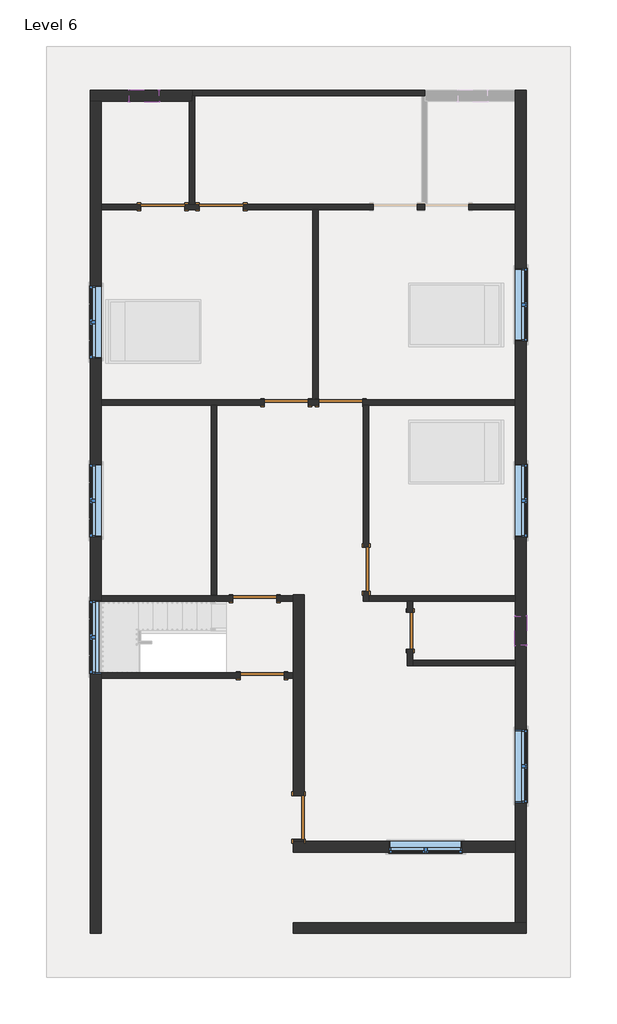
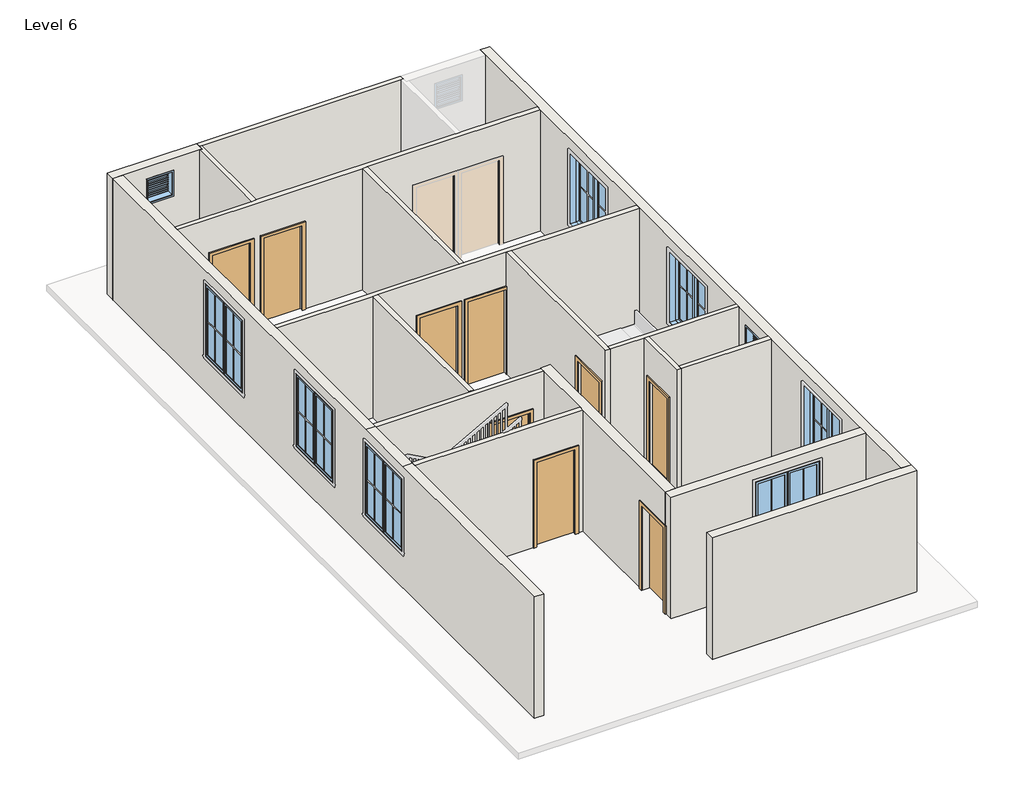
# One storey, part 1 of 3: 18 walls, 9 doors, 9 windows.
"""IFC4 building model written with IfcOpenShell, lengths in millimetres."""

from ifc_helpers import new_model, si_unit, frame, origin, place, context, project, spatial, polyline, outline, extrude, faceted_brep, transform, mapped, element, save
from components import door_78caadf7, single_flush_door_3_e5f9f3c4, single_flush_door_3_305aa2a5, single_flush_door_3_0ca8825f, window_casement_double_win_5_f93960c7, window_f2d8fef0

model = new_model("IFC4")

# Units and contexts
model_context = context("Model", 3, world=origin())
ifc_project = project(units=[si_unit("LENGTHUNIT", "METRE", prefix="MILLI")], contexts=[model_context])

# Site, building, storey
site = spatial("IfcSite", under=ifc_project)
building = spatial("IfcBuilding", under=site)
storey = spatial("IfcBuildingStorey", under=building, Name="Level 6", Elevation=12801.6)

# Doors
placement = place(None, origin())
door_shape = door_78caadf7(model_context)
element("IfcDoor", 1, ObjectType="Single-Flush : DOOR 2'6\"", at=placement, inside=storey, context=model_context, shape_type="MappedRepresentation", body=[
    mapped(door_shape, transform((860.2379845, -2779.6065691, 12801.6), x_axis=(0.0, 1.0, 0.0), y_axis=(-1.0, 0.0, 0.0), z_axis=(0.0, 0.0, 1.0))),
])
single_flush_door_3_shape = single_flush_door_3_e5f9f3c4(model_context)
element("IfcDoor", 2, ObjectType="Single-Flush : DOOR 3'", at=placement, inside=storey, context=model_context, shape_type="MappedRepresentation", body=[
    mapped(single_flush_door_3_shape, transform((-54.1620155, -1503.2565691, 12801.6), x_axis=(0.0, -1.0, 0.0), y_axis=(1.0, 0.0, 0.0), z_axis=(0.0, 0.0, 1.0))),
])
element("IfcDoor", 3, ObjectType="Single-Flush : DOOR 3'", at=placement, inside=storey, context=model_context, shape_type="MappedRepresentation", body=[
    mapped(single_flush_door_3_shape, transform((-1717.8620155, 1963.8434309, 12801.6), x_axis=(1.0, 0.0, 0.0), y_axis=(0.0, 1.0, 0.0), z_axis=(0.0, 0.0, 1.0))),
])
element("IfcDoor", 4, ObjectType="Single-Flush : DOOR 3'", at=placement, inside=storey, context=model_context, shape_type="MappedRepresentation", body=[
    mapped(single_flush_door_3_shape, transform((-2371.9120155, -2112.8565691, 12801.6), x_axis=(1.0, 0.0, 0.0), y_axis=(0.0, 1.0, 0.0), z_axis=(0.0, 0.0, 1.0))),
])
element("IfcDoor", 5, ObjectType="Single-Flush : DOOR 3'", at=placement, inside=storey, context=model_context, shape_type="MappedRepresentation", body=[
    mapped(single_flush_door_3_shape, transform((-2219.5120155, -3713.0565691, 12801.6), x_axis=(1.0, 0.0, 0.0), y_axis=(0.0, 1.0, 0.0), z_axis=(0.0, 0.0, 1.0))),
])
element("IfcDoor", 6, ObjectType="Single-Flush : DOOR 3'", at=placement, inside=storey, context=model_context, shape_type="MappedRepresentation", body=[
    mapped(single_flush_door_3_shape, transform((-4283.2620155, 6040.5434309, 12801.6), x_axis=(1.0, 0.0, 0.0), y_axis=(0.0, 1.0, 0.0), z_axis=(0.0, 0.0, 1.0))),
])
single_flush_door_3_2_shape = single_flush_door_3_305aa2a5(model_context)
element("IfcDoor", 7, ObjectType="Single-Flush : DOOR 3'", at=placement, inside=storey, context=model_context, shape_type="MappedRepresentation", body=[
    mapped(single_flush_door_3_2_shape, transform((-581.2120155, 1963.8434309, 12801.6), x_axis=(-1.0, 0.0, 0.0), y_axis=(0.0, -1.0, 0.0), z_axis=(0.0, 0.0, 1.0))),
])
element("IfcDoor", 8, ObjectType="Single-Flush : DOOR 3'", at=placement, inside=storey, context=model_context, shape_type="MappedRepresentation", body=[
    mapped(single_flush_door_3_2_shape, transform((-3064.0620155, 6040.5434309, 12801.6), x_axis=(-1.0, 0.0, 0.0), y_axis=(0.0, -1.0, 0.0), z_axis=(0.0, 0.0, 1.0))),
])
single_flush_door_3_3_shape = single_flush_door_3_0ca8825f(model_context)
element("IfcDoor", 9, ObjectType="Single-Flush : DOOR 3'", at=placement, inside=storey, context=model_context, shape_type="MappedRepresentation", body=[
    mapped(single_flush_door_3_3_shape, transform((-1457.5120155, -6665.8065691, 12801.6), x_axis=(0.0, -1.0, 0.0), y_axis=(1.0, 0.0, 0.0), z_axis=(0.0, 0.0, 1.0))),
])

# Walls
element("IfcWall", 10, ObjectType="WALL 4.5\"", at=placement, inside=storey, context=model_context, shape_type="Brep", body=[
    faceted_brep([(-3673.6620155, 8345.5934309, 12801.6), (-3616.5120155, 8345.5934309, 12801.6), (1107.8879845, 8345.5934309, 12801.6), (1165.0379845, 8345.5934309, 12801.6), (1165.0379845, 8345.5934309, 15849.6), (1107.8879845, 8345.5934309, 15849.6), (-3616.5120155, 8345.5934309, 15849.6), (-3673.6620155, 8345.5934309, 15849.6), (-3673.6620155, 8459.8934309, 12801.6), (-3673.6620155, 8459.8934309, 15849.6), (1165.0379845, 8459.8934309, 15849.6), (1165.0379845, 8459.8934309, 12801.6)], [[[0, 1, 2, 3, 4, 5, 6, 7]], [[8, 9, 10, 11]], [[3, 2, 1, 0, 8, 11]], [[4, 3, 11, 10]], [[0, 7, 9, 8]], [[7, 6, 5, 4, 10, 9]]]),
])
element("IfcWall", 11, ObjectType="WALL 4.5\"", at=placement, inside=storey, context=model_context, shape_type="SweptSolid", body=[
    extrude(outline(polyline([(-3730.8120155, 6097.6934309), (-3730.8120155, 8231.2934309), (-3673.6620155, 8231.2934309), (-3673.6620155, 8345.5934309), (-3616.5120155, 8345.5934309), (-3616.5120155, 6097.6934309), (-3730.8120155, 6097.6934309)])), frame((0.0, 0.0, 12801.6), z_axis=(0.0, 0.0, 1.0), x_axis=(1.0, 0.0, 0.0)), (0.0, 0.0, 1.0), 3048.0),
])
element("IfcWall", 12, ObjectType="WALL 4.5\"", at=placement, inside=storey, context=model_context, shape_type="Brep", body=[
    faceted_brep([(1165.0379845, 6097.6934309, 14935.2), (1165.0379845, 6097.6934309, 12801.6), (1107.8879845, 6097.6934309, 12801.6), (1012.6379845, 6097.6934309, 12801.6), (1012.6379845, 6097.6934309, 14935.2), (98.2379845, 6097.6934309, 14935.2), (98.2379845, 6097.6934309, 12801.6), (-2606.8620155, 6097.6934309, 12801.6), (-2606.8620155, 6097.6934309, 14935.2), (-3521.2620155, 6097.6934309, 14935.2), (-3521.2620155, 6097.6934309, 12801.6), (-3616.5120155, 6097.6934309, 12801.6), (-3730.8120155, 6097.6934309, 12801.6), (-3826.0620155, 6097.6934309, 12801.6), (-3826.0620155, 6097.6934309, 14935.2), (-4740.4620155, 6097.6934309, 14935.2), (-4740.4620155, 6097.6934309, 12801.6), (-5559.6120155, 6097.6934309, 12801.6), (-5559.6120155, 6097.6934309, 15849.6), (-3730.8120155, 6097.6934309, 15849.6), (-3616.5120155, 6097.6934309, 15849.6), (1107.8879845, 6097.6934309, 15849.6), (1222.1879845, 6097.6934309, 15849.6), (3050.9879845, 6097.6934309, 15849.6), (3050.9879845, 6097.6934309, 12801.6), (2079.4379845, 6097.6934309, 12801.6), (2079.4379845, 6097.6934309, 14935.2), (1012.6379845, 5983.3934309, 12801.6), (1165.0379845, 5983.3934309, 12801.6), (1165.0379845, 5983.3934309, 14935.2), (2079.4379845, 5983.3934309, 14935.2), (2079.4379845, 5983.3934309, 12801.6), (3050.9879845, 5983.3934309, 12801.6), (3050.9879845, 5983.3934309, 15849.6), (-1051.1120155, 5983.3934309, 15849.6), (-1165.4120155, 5983.3934309, 15849.6), (-5559.6120155, 5983.3934309, 15849.6), (-5559.6120155, 5983.3934309, 12801.6), (-4740.4620155, 5983.3934309, 12801.6), (-4740.4620155, 5983.3934309, 14935.2), (-3826.0620155, 5983.3934309, 14935.2), (-3826.0620155, 5983.3934309, 12801.6), (-3521.2620155, 5983.3934309, 12801.6), (-3521.2620155, 5983.3934309, 14935.2), (-2606.8620155, 5983.3934309, 14935.2), (-2606.8620155, 5983.3934309, 12801.6), (-1165.4120155, 5983.3934309, 12801.6), (-1051.1120155, 5983.3934309, 12801.6), (98.2379845, 5983.3934309, 12801.6), (98.2379845, 5983.3934309, 14935.2), (1012.6379845, 5983.3934309, 14935.2)], [[[0, 1, 2, 3, 4, 5, 6, 7, 8, 9, 10, 11, 12, 13, 14, 15, 16, 17, 18, 19, 20, 21, 22, 23, 24, 25, 26]], [[27, 28, 29, 30, 31, 32, 33, 34, 35, 36, 37, 38, 39, 40, 41, 42, 43, 44, 45, 46, 47, 48, 49, 50]], [[38, 37, 17, 16]], [[13, 12, 11, 10, 42, 41]], [[48, 47, 46, 45, 7, 6]], [[25, 24, 32, 31]], [[3, 2, 1, 28, 27]], [[18, 17, 37, 36]], [[24, 23, 33, 32]], [[14, 13, 41, 40]], [[15, 14, 40, 39]], [[16, 15, 39, 38]], [[43, 42, 10, 9]], [[44, 43, 9, 8]], [[45, 44, 8, 7]], [[4, 3, 27, 50]], [[5, 4, 50, 49]], [[6, 5, 49, 48]], [[29, 28, 1, 0]], [[30, 29, 0, 26]], [[31, 30, 26, 25]], [[23, 22, 21, 20, 19, 18, 36, 35, 34, 33]]]),
])
element("IfcWall", 13, ObjectType="WALL 4.5\"", at=placement, inside=storey, context=model_context, shape_type="SweptSolid", body=[
    extrude(outline(polyline([(-1165.4120155, 2020.9934309), (-1165.4120155, 5983.3934309), (-1051.1120155, 5983.3934309), (-1051.1120155, 2020.9934309), (-1165.4120155, 2020.9934309)])), frame((0.0, 0.0, 12801.6), z_axis=(0.0, 0.0, 1.0), x_axis=(1.0, 0.0, 0.0)), (0.0, 0.0, 1.0), 3048.0),
])
element("IfcWall", 14, ObjectType="WALL 4.5\"", at=placement, inside=storey, context=model_context, shape_type="Brep", body=[
    faceted_brep([(-1260.6620155, 1906.6934309, 14935.2), (-1260.6620155, 1906.6934309, 12801.6), (-1038.4120155, 1906.6934309, 12801.6), (-1038.4120155, 1906.6934309, 14935.2), (-124.0120155, 1906.6934309, 14935.2), (-124.0120155, 1906.6934309, 12801.6), (-111.3120155, 1906.6934309, 12801.6), (2.9879845, 1906.6934309, 12801.6), (3050.9879845, 1906.6934309, 12801.6), (3050.9879845, 1906.6934309, 15849.6), (2.9879845, 1906.6934309, 15849.6), (-111.3120155, 1906.6934309, 15849.6), (-3159.3120155, 1906.6934309, 15849.6), (-3273.6120155, 1906.6934309, 15849.6), (-5559.6120155, 1906.6934309, 15849.6), (-5559.6120155, 1906.6934309, 12801.6), (-3273.6120155, 1906.6934309, 12801.6), (-3159.3120155, 1906.6934309, 12801.6), (-2175.0620155, 1906.6934309, 12801.6), (-2175.0620155, 1906.6934309, 14935.2), (-1038.4120155, 2020.9934309, 12801.6), (-1051.1120155, 2020.9934309, 12801.6), (-1165.4120155, 2020.9934309, 12801.6), (-1260.6620155, 2020.9934309, 12801.6), (-1260.6620155, 2020.9934309, 14935.2), (-2175.0620155, 2020.9934309, 14935.2), (-2175.0620155, 2020.9934309, 12801.6), (-5559.6120155, 2020.9934309, 12801.6), (-5559.6120155, 2020.9934309, 15849.6), (-1165.4120155, 2020.9934309, 15849.6), (-1051.1120155, 2020.9934309, 15849.6), (3050.9879845, 2020.9934309, 15849.6), (3050.9879845, 2020.9934309, 12801.6), (-124.0120155, 2020.9934309, 12801.6), (-124.0120155, 2020.9934309, 14935.2), (-1038.4120155, 2020.9934309, 14935.2)], [[[0, 1, 2, 3, 4, 5, 6, 7, 8, 9, 10, 11, 12, 13, 14, 15, 16, 17, 18, 19]], [[20, 21, 22, 23, 24, 25, 26, 27, 28, 29, 30, 31, 32, 33, 34, 35]], [[33, 32, 8, 7, 6, 5]], [[2, 1, 23, 22, 21, 20]], [[18, 17, 16, 15, 27, 26]], [[15, 14, 28, 27]], [[9, 8, 32, 31]], [[3, 2, 20, 35]], [[4, 3, 35, 34]], [[5, 4, 34, 33]], [[24, 23, 1, 0]], [[25, 24, 0, 19]], [[26, 25, 19, 18]], [[14, 13, 12, 11, 10, 9, 31, 30, 29, 28]]]),
])
element("IfcWall", 15, ObjectType="WALL 4.5\"", at=placement, inside=storey, context=model_context, shape_type="SweptSolid", body=[
    extrude(outline(polyline([(-3273.6120155, -2032.8465691), (-3273.6120155, 1906.6934309), (-3159.3120155, 1906.6934309), (-3159.3120155, -2032.8465691), (-3273.6120155, -2032.8465691)])), frame((0.0, 0.0, 12801.6), z_axis=(0.0, 0.0, 1.0), x_axis=(1.0, 0.0, 0.0)), (0.0, 0.0, 1.0), 3048.0),
])
element("IfcWall", 16, ObjectType="WALL 4.5\"", at=placement, inside=storey, context=model_context, shape_type="SweptSolid", body=[
    extrude(outline(polyline([(14935.2, -1914.7120155), (12801.6, -1914.7120155), (12801.6, -1571.8120155), (15849.6, -1571.8120155), (15849.6, -5559.6120155), (12801.6, -5559.6120155), (12801.6, -2829.1120155), (14935.2, -2829.1120155), (14935.2, -1914.7120155)])), frame((0.0, -2170.0065691, 0.0), z_axis=(0.0, 1.0, 0.0), x_axis=(0.0, 0.0, 1.0)), (0.0, 0.0, 1.0), 114.3),
])
element("IfcWall", 17, ObjectType="WALL 4.5\"", at=placement, inside=storey, context=model_context, shape_type="SweptSolid", body=[
    extrude(outline(polyline([(14935.2, -1762.3120155), (12801.6, -1762.3120155), (12801.6, -1571.8120155), (15849.6, -1571.8120155), (15849.6, -5559.6120155), (12801.6, -5559.6120155), (12801.6, -2676.7120155), (14935.2, -2676.7120155), (14935.2, -1762.3120155)])), frame((0.0, -3770.2065691, 0.0), z_axis=(0.0, 1.0, 0.0), x_axis=(0.0, 0.0, 1.0)), (0.0, 0.0, 1.0), 114.3),
])
element("IfcWall", 18, ObjectType="WALL 4.5\"", at=placement, inside=storey, context=model_context, shape_type="Brep", body=[
    faceted_brep([(-111.3120155, -1960.4565691, 14935.2), (-111.3120155, -1960.4565691, 12801.6), (-111.3120155, -2170.0065691, 12801.6), (-111.3120155, -2170.0065691, 15849.6), (-111.3120155, 1906.6934309, 15849.6), (-111.3120155, 1906.6934309, 12801.6), (-111.3120155, -1046.0565691, 12801.6), (-111.3120155, -1046.0565691, 14935.2), (2.9879845, -2170.0065691, 12801.6), (2.9879845, -2055.7065691, 12801.6), (2.9879845, -1960.4565691, 12801.6), (2.9879845, -1960.4565691, 14935.2), (2.9879845, -1046.0565691, 14935.2), (2.9879845, -1046.0565691, 12801.6), (2.9879845, 1906.6934309, 12801.6), (2.9879845, 1906.6934309, 15849.6), (2.9879845, -2055.7065691, 15849.6), (2.9879845, -2170.0065691, 15849.6)], [[[0, 1, 2, 3, 4, 5, 6, 7]], [[8, 9, 10, 11, 12, 13, 14, 15, 16, 17]], [[6, 5, 14, 13]], [[2, 1, 10, 9, 8]], [[5, 4, 15, 14]], [[3, 2, 8, 17]], [[11, 10, 1, 0]], [[12, 11, 0, 7]], [[13, 12, 7, 6]], [[4, 3, 17, 16, 15]]]),
])
element("IfcWall", 19, ObjectType="WALL 4.5\"", at=placement, inside=storey, context=model_context, shape_type="Brep", body=[
    faceted_brep([(2.9879845, -2170.0065691, 12801.6), (803.0879845, -2170.0065691, 12801.6), (917.3879845, -2170.0065691, 12801.6), (3050.9879845, -2170.0065691, 12801.6), (3050.9879845, -2170.0065691, 15849.6), (917.3879845, -2170.0065691, 15849.6), (803.0879845, -2170.0065691, 15849.6), (2.9879845, -2170.0065691, 15849.6), (2.9879845, -2055.7065691, 12801.6), (2.9879845, -2055.7065691, 15849.6), (3050.9879845, -2055.7065691, 15849.6), (3050.9879845, -2055.7065691, 12801.6)], [[[0, 1, 2, 3, 4, 5, 6, 7]], [[8, 9, 10, 11]], [[3, 2, 1, 0, 8, 11]], [[0, 7, 9, 8]], [[4, 3, 11, 10]], [[7, 6, 5, 4, 10, 9]]]),
])
element("IfcWall", 20, ObjectType="WALL 4.5\"", at=placement, inside=storey, context=model_context, shape_type="Brep", body=[
    faceted_brep([(803.0879845, -2170.0065691, 12801.6), (803.0879845, -2398.6065691, 12801.6), (803.0879845, -2398.6065691, 14935.2), (803.0879845, -3160.6065691, 14935.2), (803.0879845, -3160.6065691, 12801.6), (803.0879845, -3503.5065691, 12801.6), (803.0879845, -3503.5065691, 15849.6), (803.0879845, -2170.0065691, 15849.6), (917.3879845, -2398.6065691, 14935.2), (917.3879845, -2398.6065691, 12801.6), (917.3879845, -2170.0065691, 12801.6), (917.3879845, -2170.0065691, 15849.6), (917.3879845, -3389.2065691, 15849.6), (917.3879845, -3503.5065691, 15849.6), (917.3879845, -3503.5065691, 12801.6), (917.3879845, -3389.2065691, 12801.6), (917.3879845, -3160.6065691, 12801.6), (917.3879845, -3160.6065691, 14935.2)], [[[0, 1, 2, 3, 4, 5, 6, 7]], [[8, 9, 10, 11, 12, 13, 14, 15, 16, 17]], [[10, 9, 1, 0]], [[16, 15, 14, 5, 4]], [[0, 7, 11, 10]], [[6, 5, 14, 13]], [[2, 1, 9, 8]], [[3, 2, 8, 17]], [[4, 3, 17, 16]], [[7, 6, 13, 12, 11]]]),
])
element("IfcWall", 21, ObjectType="WALL 4.5\"", at=placement, inside=storey, context=model_context, shape_type="SweptSolid", body=[
    extrude(outline(polyline([(917.3879845, -3389.2065691), (3050.9879845, -3389.2065691), (3050.9879845, -3503.5065691), (917.3879845, -3503.5065691), (917.3879845, -3389.2065691)])), frame((0.0, 0.0, 12801.6), z_axis=(0.0, 0.0, 1.0), x_axis=(1.0, 0.0, 0.0)), (0.0, 0.0, 1.0), 3048.0),
])
element("IfcWall", 22, ObjectType="WALL 9\"", at=placement, inside=storey, context=model_context, shape_type="Brep", body=[
    faceted_brep([(-3673.6620155, 8459.8934309, 12801.6), (-5788.2120155, 8459.8934309, 12801.6), (-5788.2120155, 8459.8934309, 15849.6), (-3673.6620155, 8459.8934309, 15849.6), (-4978.5870155, 8459.8934309, 15544.8), (-4978.5870155, 8459.8934309, 14935.2), (-4368.9870155, 8459.8934309, 14935.2), (-4368.9870155, 8459.8934309, 15544.8), (-3673.6620155, 8231.2934309, 12801.6), (-3673.6620155, 8231.2934309, 15849.6), (-3730.8120155, 8231.2934309, 15849.6), (-5559.6120155, 8231.2934309, 15849.6), (-5788.2120155, 8231.2934309, 15849.6), (-5788.2120155, 8231.2934309, 12801.6), (-5559.6120155, 8231.2934309, 12801.6), (-3730.8120155, 8231.2934309, 12801.6), (-4978.5870155, 8231.2934309, 15544.8), (-4368.9870155, 8231.2934309, 15544.8), (-4368.9870155, 8231.2934309, 14935.2), (-4978.5870155, 8231.2934309, 14935.2), (-3673.6620155, 8345.5934309, 12801.6), (-3673.6620155, 8345.5934309, 15849.6)], [[[0, 1, 2, 3], [4, 5, 6, 7]], [[8, 9, 10, 11, 12, 13, 14, 15], [16, 17, 18, 19]], [[1, 0, 20, 8, 15, 14, 13]], [[0, 3, 21, 9, 8, 20]], [[2, 1, 13, 12]], [[5, 4, 16, 19]], [[6, 5, 19, 18]], [[7, 6, 18, 17]], [[4, 7, 17, 16]], [[3, 2, 12, 11, 10, 9, 21]]]),
])
element("IfcWall", 23, ObjectType="WALL 9\"", at=placement, inside=storey, context=model_context, shape_type="Brep", body=[
    faceted_brep([(-5788.2120155, 8231.2934309, 12801.6), (-5788.2120155, -9078.8065691, 12801.6), (-5788.2120155, -9078.8065691, 15849.6), (-5788.2120155, -3674.9565691, 15849.6), (-5788.2120155, -2150.9565691, 15849.6), (-5788.2120155, 8231.2934309, 15849.6), (-5788.2120155, 4402.2434309, 15544.8), (-5788.2120155, 2878.2434309, 15544.8), (-5788.2120155, 2878.2434309, 13716.0), (-5788.2120155, 4402.2434309, 13716.0), (-5788.2120155, -2150.9565691, 15544.8), (-5788.2120155, -3674.9565691, 15544.8), (-5788.2120155, -3674.9565691, 13716.0), (-5788.2120155, -2150.9565691, 13716.0), (-5788.2120155, 687.4934309, 15544.8), (-5788.2120155, -836.5065691, 15544.8), (-5788.2120155, -836.5065691, 13716.0), (-5788.2120155, 687.4934309, 13716.0), (-5559.6120155, 8231.2934309, 12801.6), (-5559.6120155, 8231.2934309, 15849.6), (-5559.6120155, 6097.6934309, 15849.6), (-5559.6120155, 5983.3934309, 15849.6), (-5559.6120155, 2020.9934309, 15849.6), (-5559.6120155, 1906.6934309, 15849.6), (-5559.6120155, -2055.7065691, 15849.6), (-5559.6120155, -2150.9565691, 15849.6), (-5559.6120155, -2170.0065691, 15849.6), (-5559.6120155, -3655.9065691, 15849.6), (-5559.6120155, -3674.9565691, 15849.6), (-5559.6120155, -3770.2065691, 15849.6), (-5559.6120155, -9078.8065691, 15849.6), (-5559.6120155, -9078.8065691, 12801.6), (-5559.6120155, -3770.2065691, 12801.6), (-5559.6120155, -3655.9065691, 12801.6), (-5559.6120155, -2170.0065691, 12801.6), (-5559.6120155, -2055.7065691, 12801.6), (-5559.6120155, 1906.6934309, 12801.6), (-5559.6120155, 2020.9934309, 12801.6), (-5559.6120155, 5983.3934309, 12801.6), (-5559.6120155, 6097.6934309, 12801.6), (-5559.6120155, 4402.2434309, 15544.8), (-5559.6120155, 4402.2434309, 13716.0), (-5559.6120155, 2878.2434309, 13716.0), (-5559.6120155, 2878.2434309, 15544.8), (-5559.6120155, -2150.9565691, 15544.8), (-5559.6120155, -2150.9565691, 13716.0), (-5559.6120155, -3674.9565691, 13716.0), (-5559.6120155, -3674.9565691, 15544.8), (-5559.6120155, 687.4934309, 15544.8), (-5559.6120155, 687.4934309, 13716.0), (-5559.6120155, -836.5065691, 13716.0), (-5559.6120155, -836.5065691, 15544.8)], [[[0, 1, 2, 3, 4, 5], [6, 7, 8, 9], [10, 11, 12, 13], [14, 15, 16, 17]], [[18, 19, 20, 21, 22, 23, 24, 25, 26, 27, 28, 29, 30, 31, 32, 33, 34, 35, 36, 37, 38, 39], [40, 41, 42, 43], [44, 45, 46, 47], [48, 49, 50, 51]], [[1, 0, 18, 39, 38, 37, 36, 35, 34, 33, 32, 31]], [[2, 1, 31, 30]], [[0, 5, 19, 18]], [[41, 40, 6, 9]], [[42, 41, 9, 8]], [[43, 42, 8, 7]], [[40, 43, 7, 6]], [[45, 44, 10, 13]], [[46, 45, 13, 12]], [[47, 46, 12, 11]], [[44, 47, 11, 10]], [[49, 48, 14, 17]], [[50, 49, 17, 16]], [[51, 50, 16, 15]], [[48, 51, 15, 14]], [[4, 3, 28, 27, 26, 25]], [[3, 2, 30, 29, 28]], [[5, 4, 25, 24, 23, 22, 21, 20, 19]]]),
])
element("IfcWall", 24, ObjectType="WALL 9\"", at=placement, inside=storey, context=model_context, shape_type="Brep", body=[
    faceted_brep([(-1571.8120155, -9078.8065691, 12801.6), (3279.5879845, -9078.8065691, 12801.6), (3279.5879845, -9078.8065691, 15849.6), (-1571.8120155, -9078.8065691, 15849.6), (-1571.8120155, -8850.2065691, 12801.6), (-1571.8120155, -8850.2065691, 15849.6), (3050.9879845, -8850.2065691, 15849.6), (3279.5879845, -8850.2065691, 15849.6), (3279.5879845, -8850.2065691, 12801.6), (3050.9879845, -8850.2065691, 12801.6)], [[[0, 1, 2, 3]], [[4, 5, 6, 7, 8, 9]], [[1, 0, 4, 9, 8]], [[0, 3, 5, 4]], [[2, 1, 8, 7]], [[3, 2, 7, 6, 5]]]),
])
element("IfcWall", 25, ObjectType="WALL 9\"", at=placement, inside=storey, context=model_context, shape_type="Brep", body=[
    faceted_brep([(3279.5879845, -8850.2065691, 12801.6), (3279.5879845, 8459.8934309, 12801.6), (3279.5879845, 8459.8934309, 15849.6), (3279.5879845, -8850.2065691, 15849.6), (3279.5879845, 3240.1934309, 15544.8), (3279.5879845, 4764.1934309, 15544.8), (3279.5879845, 4764.1934309, 13716.0), (3279.5879845, 3240.1934309, 13716.0), (3279.5879845, -836.5065691, 15544.8), (3279.5879845, 687.4934309, 15544.8), (3279.5879845, 687.4934309, 13716.0), (3279.5879845, -836.5065691, 13716.0), (3279.5879845, -6361.0065691, 15544.8), (3279.5879845, -4837.0065691, 15544.8), (3279.5879845, -4837.0065691, 13716.0), (3279.5879845, -6361.0065691, 13716.0), (3279.5879845, -2474.8065691, 15544.8), (3279.5879845, -2474.8065691, 14935.2), (3279.5879845, -3084.4065691, 14935.2), (3279.5879845, -3084.4065691, 15544.8), (3050.9879845, -8850.2065691, 12801.6), (3050.9879845, -8850.2065691, 15849.6), (3050.9879845, -7389.7065691, 15849.6), (3050.9879845, -7161.1065691, 15849.6), (3050.9879845, -3503.5065691, 15849.6), (3050.9879845, -3389.2065691, 15849.6), (3050.9879845, -2170.0065691, 15849.6), (3050.9879845, -2055.7065691, 15849.6), (3050.9879845, 1906.6934309, 15849.6), (3050.9879845, 2020.9934309, 15849.6), (3050.9879845, 5983.3934309, 15849.6), (3050.9879845, 6097.6934309, 15849.6), (3050.9879845, 8231.2934309, 15849.6), (3050.9879845, 8459.8934309, 15849.6), (3050.9879845, 8459.8934309, 12801.6), (3050.9879845, 8231.2934309, 12801.6), (3050.9879845, 6097.6934309, 12801.6), (3050.9879845, 5983.3934309, 12801.6), (3050.9879845, 2020.9934309, 12801.6), (3050.9879845, 1906.6934309, 12801.6), (3050.9879845, -2055.7065691, 12801.6), (3050.9879845, -2170.0065691, 12801.6), (3050.9879845, -3389.2065691, 12801.6), (3050.9879845, -3503.5065691, 12801.6), (3050.9879845, -7161.1065691, 12801.6), (3050.9879845, -7389.7065691, 12801.6), (3050.9879845, 3240.1934309, 15544.8), (3050.9879845, 3240.1934309, 13716.0), (3050.9879845, 4764.1934309, 13716.0), (3050.9879845, 4764.1934309, 15544.8), (3050.9879845, -836.5065691, 15544.8), (3050.9879845, -836.5065691, 13716.0), (3050.9879845, 687.4934309, 13716.0), (3050.9879845, 687.4934309, 15544.8), (3050.9879845, -6361.0065691, 15544.8), (3050.9879845, -6361.0065691, 13716.0), (3050.9879845, -4837.0065691, 13716.0), (3050.9879845, -4837.0065691, 15544.8), (3050.9879845, -2474.8065691, 15544.8), (3050.9879845, -3084.4065691, 15544.8), (3050.9879845, -3084.4065691, 14935.2), (3050.9879845, -2474.8065691, 14935.2)], [[[0, 1, 2, 3], [4, 5, 6, 7], [8, 9, 10, 11], [12, 13, 14, 15], [16, 17, 18, 19]], [[20, 21, 22, 23, 24, 25, 26, 27, 28, 29, 30, 31, 32, 33, 34, 35, 36, 37, 38, 39, 40, 41, 42, 43, 44, 45], [46, 47, 48, 49], [50, 51, 52, 53], [54, 55, 56, 57], [58, 59, 60, 61]], [[1, 0, 20, 45, 44, 43, 42, 41, 40, 39, 38, 37, 36, 35, 34]], [[0, 3, 21, 20]], [[2, 1, 34, 33]], [[47, 46, 4, 7]], [[48, 47, 7, 6]], [[49, 48, 6, 5]], [[46, 49, 5, 4]], [[51, 50, 8, 11]], [[52, 51, 11, 10]], [[53, 52, 10, 9]], [[50, 53, 9, 8]], [[55, 54, 12, 15]], [[56, 55, 15, 14]], [[57, 56, 14, 13]], [[54, 57, 13, 12]], [[17, 16, 58, 61]], [[18, 17, 61, 60]], [[19, 18, 60, 59]], [[16, 19, 59, 58]], [[3, 2, 33, 32, 31, 30, 29, 28, 27, 26, 25, 24, 23, 22, 21]]]),
])
element("IfcWall", 26, ObjectType="WALL 9\"", at=placement, inside=storey, context=model_context, shape_type="Brep", body=[
    faceted_brep([(3050.9879845, -7161.1065691, 12801.6), (-1343.2120155, -7161.1065691, 12801.6), (-1571.8120155, -7161.1065691, 12801.6), (-1571.8120155, -7161.1065691, 15849.6), (-1343.2120155, -7161.1065691, 15849.6), (3050.9879845, -7161.1065691, 15849.6), (422.0879845, -7161.1065691, 15544.8), (422.0879845, -7161.1065691, 13716.0), (1946.0879845, -7161.1065691, 13716.0), (1946.0879845, -7161.1065691, 15544.8), (3050.9879845, -7389.7065691, 12801.6), (3050.9879845, -7389.7065691, 15849.6), (-1571.8120155, -7389.7065691, 15849.6), (-1571.8120155, -7389.7065691, 12801.6), (422.0879845, -7389.7065691, 15544.8), (1946.0879845, -7389.7065691, 15544.8), (1946.0879845, -7389.7065691, 13716.0), (422.0879845, -7389.7065691, 13716.0)], [[[0, 1, 2, 3, 4, 5], [6, 7, 8, 9]], [[10, 11, 12, 13], [14, 15, 16, 17]], [[2, 1, 0, 10, 13]], [[0, 5, 11, 10]], [[3, 2, 13, 12]], [[7, 6, 14, 17]], [[8, 7, 17, 16]], [[9, 8, 16, 15]], [[6, 9, 15, 14]], [[5, 4, 3, 12, 11]]]),
])
element("IfcWall", 27, ObjectType="WALL 9\"", at=placement, inside=storey, context=model_context, shape_type="Brep", body=[
    faceted_brep([(-1343.2120155, -7161.1065691, 12801.6), (-1343.2120155, -7123.0065691, 12801.6), (-1343.2120155, -7123.0065691, 14935.2), (-1343.2120155, -6208.6065691, 14935.2), (-1343.2120155, -6208.6065691, 12801.6), (-1343.2120155, -2032.8465691, 12801.6), (-1343.2120155, -2032.8465691, 15849.6), (-1343.2120155, -7161.1065691, 15849.6), (-1571.8120155, -7123.0065691, 14935.2), (-1571.8120155, -7123.0065691, 12801.6), (-1571.8120155, -7161.1065691, 12801.6), (-1571.8120155, -7161.1065691, 15849.6), (-1571.8120155, -3770.2065691, 15849.6), (-1571.8120155, -3655.9065691, 15849.6), (-1571.8120155, -2170.0065691, 15849.6), (-1571.8120155, -2055.7065691, 15849.6), (-1571.8120155, -2032.8465691, 15849.6), (-1571.8120155, -2032.8465691, 12801.6), (-1571.8120155, -2055.7065691, 12801.6), (-1571.8120155, -2170.0065691, 12801.6), (-1571.8120155, -3655.9065691, 12801.6), (-1571.8120155, -3770.2065691, 12801.6), (-1571.8120155, -6208.6065691, 12801.6), (-1571.8120155, -6208.6065691, 14935.2)], [[[0, 1, 2, 3, 4, 5, 6, 7]], [[8, 9, 10, 11, 12, 13, 14, 15, 16, 17, 18, 19, 20, 21, 22, 23]], [[10, 9, 1, 0]], [[22, 21, 20, 19, 18, 17, 5, 4]], [[6, 5, 17, 16]], [[0, 7, 11, 10]], [[2, 1, 9, 8]], [[3, 2, 8, 23]], [[4, 3, 23, 22]], [[7, 6, 16, 15, 14, 13, 12, 11]]]),
])

# Windows
window_casement_double_win_5_shape = window_casement_double_win_5_f93960c7(model_context)
element("IfcWindow", 28, ObjectType="Window-Casement-Double : WIN 5'", at=placement, inside=storey, context=model_context, shape_type="MappedRepresentation", body=[
    mapped(window_casement_double_win_5_shape, transform((-5673.9120155, 3640.2434309, 12801.6), x_axis=(0.0, 1.0, 0.0), y_axis=(-1.0, 0.0, 0.0), z_axis=(0.0, 0.0, 1.0))),
])
element("IfcWindow", 29, ObjectType="Window-Casement-Double : WIN 5'", at=placement, inside=storey, context=model_context, shape_type="MappedRepresentation", body=[
    mapped(window_casement_double_win_5_shape, transform((3165.2879845, 4002.1934309, 12801.6), x_axis=(0.0, -1.0, 0.0), y_axis=(1.0, 0.0, 0.0), z_axis=(0.0, 0.0, 1.0))),
])
element("IfcWindow", 30, ObjectType="Window-Casement-Double : WIN 5'", at=placement, inside=storey, context=model_context, shape_type="MappedRepresentation", body=[
    mapped(window_casement_double_win_5_shape, transform((3165.2879845, -74.5065691, 12801.6), x_axis=(0.0, -1.0, 0.0), y_axis=(1.0, 0.0, 0.0), z_axis=(0.0, 0.0, 1.0))),
])
element("IfcWindow", 31, ObjectType="Window-Casement-Double : WIN 5'", at=placement, inside=storey, context=model_context, shape_type="MappedRepresentation", body=[
    mapped(window_casement_double_win_5_shape, transform((3165.2879845, -5599.0065691, 12801.6), x_axis=(0.0, -1.0, 0.0), y_axis=(1.0, 0.0, 0.0), z_axis=(0.0, 0.0, 1.0))),
])
element("IfcWindow", 32, ObjectType="Window-Casement-Double : WIN 5'", at=placement, inside=storey, context=model_context, shape_type="MappedRepresentation", body=[
    mapped(window_casement_double_win_5_shape, transform((1184.0879845, -7275.4065691, 12801.6), x_axis=(-1.0, 0.0, 0.0), y_axis=(0.0, -1.0, 0.0), z_axis=(0.0, 0.0, 1.0))),
])
element("IfcWindow", 33, ObjectType="Window-Casement-Double : WIN 5'", at=placement, inside=storey, context=model_context, shape_type="MappedRepresentation", body=[
    mapped(window_casement_double_win_5_shape, transform((-5673.9120155, -2912.9565691, 12801.6), x_axis=(0.0, 1.0, 0.0), y_axis=(-1.0, 0.0, 0.0), z_axis=(0.0, 0.0, 1.0))),
])
element("IfcWindow", 34, ObjectType="Window-Casement-Double : WIN 5'", at=placement, inside=storey, context=model_context, shape_type="MappedRepresentation", body=[
    mapped(window_casement_double_win_5_shape, transform((-5673.9120155, -74.5065691, 12801.6), x_axis=(0.0, 1.0, 0.0), y_axis=(-1.0, 0.0, 0.0), z_axis=(0.0, 0.0, 1.0))),
])
window_shape = window_f2d8fef0(model_context)
element("IfcWindow", 35, ObjectType="Window-Louvers : 24\" x 24\"", at=placement, inside=storey, context=model_context, shape_type="MappedRepresentation", body=[
    mapped(window_shape, transform((-4673.7870155, 8351.9434309, 14020.8), x_axis=(1.0, 0.0, 0.0), y_axis=(0.0, 1.0, 0.0), z_axis=(0.0, 0.0, 1.0))),
])
element("IfcWindow", 36, ObjectType="Window-Louvers : 24\" x 24\"", at=placement, inside=storey, context=model_context, shape_type="MappedRepresentation", body=[
    mapped(window_shape, transform((3171.6379845, -2779.6065691, 14020.8), x_axis=(0.0, -1.0, 0.0), y_axis=(1.0, 0.0, 0.0), z_axis=(0.0, 0.0, 1.0))),
])

save(model, "model.ifc")

# Revit data of these elements
# Type "Single-Flush : DOOR 2'6\""
#   Type Mark = "10"
#   Construction Type Id = "MDOOR"
#   Assembly Code = "C1020"
#   Analytic Construction = "Metal"
#   Thickness = 0' - 2"
#   Heat Transfer Coefficient (U) = 0.651978 BTU/(h·ft²·°F)
#   Height = 7' - 0"
#   Trim Projection Ext = 0' - 1"
#   Trim Projection Int = 0' - 1"
#   Trim Width = 0' - 3"
#   Width = 2' - 6"
#   Define Thermal Properties by = 1
#   Door Material = Door - Panel
#   Frame Material = Door - Frame
#   Visual Light Transmittance = 0
#   Solar Heat Gain Coefficient = 0
#   Function = (empty or 0)
#   Wall Closure = (empty or 0)
# Type "Single-Flush : DOOR 3'"
#   Type Mark = "9"
#   Construction Type Id = "MDOOR"
#   Assembly Code = "C1020"
#   Analytic Construction = "Metal"
#   Thickness = 0' - 2"
#   Heat Transfer Coefficient (U) = 0.651978 BTU/(h·ft²·°F)
#   Height = 7' - 0"
#   Trim Projection Ext = 0' - 1"
#   Trim Projection Int = 0' - 1"
#   Trim Width = 0' - 3"
#   Width = 3' - 0"
#   Define Thermal Properties by = 1
#   Door Material = Door - Panel
#   Frame Material = Door - Frame
#   Visual Light Transmittance = 0
#   Solar Heat Gain Coefficient = 0
#   Function = (empty or 0)
#   Wall Closure = (empty or 0)
# Type "WALL 4.5\""
#   Assembly Code = "B2010"
#   Layers, outside or top first: 0' - 4 1/2" no material (function 1)
# Type "WALL 9\""
#   Assembly Code = "B2010"
#   Layers, outside or top first: 0' - 9" no material (function 1)
# Type "Window-Casement-Double : WIN 5'"
#   Type Mark = "18"
#   Fire Rating = "0.5h"
#   Assembly Code = "B2020100"
#   Analytic Construction = "Double glazing - domestic"
#   Frame Extension [instance default] = 0' - 0 1/4"
#   Window Inset [instance default] = 0' - 0"
#   Wall Thickness [instance default] = 0' - 6"
#   Interior Wall Closure [instance default] = 0' - 2 1/4"
#   Half Width = 2' - 6"
#   Visual Light Transmittance = 0.81
#   Thermal Resistance (R) = 1.8146 (h·ft²·°F)/BTU
#   Solar Heat Gain Coefficient = 0.76
#   Rough Width = 5' - 0 1/2"
#   Rough Height = 6' - 0 1/2"
#   Height = 6' - 0"
#   Heat Transfer Coefficient (U) = 0.5511 BTU/(h·ft²·°F)
#   Exterior Wall Closure [instance default] = 0' - 1 1/4"
#   Extension Jamb [instance default] = 0' - 2 1/4"
#   Default Sill Height = 3' - 0"
#   Width = 5' - 0"
#   Muntin Visibility = yes
#   Interior Trim Visibility [instance default] = yes
#   Exterior Trim Visibility [instance default] = yes
#   Extension Jamb Visibility [instance default] = yes
#   Interior Trim Material = Wood - Stained
#   Muntin Pattern = Muntin Pattern_2x2 : Muntin Pattern_2x2
#   Interior Trim = Trim-Window-Interior-Flat : Picture Frame
#   Interior Frame Material = Wood - Stained
#   Glass Panel Material = Glass
#   Exterior Trim Material = Clad - White
#   Exterior Trim = Trim-Window-Exterior-Flat : with Sill
#   Exterior Frame Material = Clad - White
#   Wall Closure = (empty or 0)
# Type "Window-Louvers : 24\" x 24\""
#   Type Mark = "19"
#   Construction Type Id = "GSP4R"
#   Assembly Code = "B20"
#   Analytic Construction = "1/8 in Pilkington single glazing"
#   Visual Light Transmittance = 0.9
#   Thermal Resistance (R) = 1.53941 (h·ft²·°F)/BTU
#   Solar Heat Gain Coefficient = 0.78
#   Max Height = 1' - 11.74264"
#   Height = 2' - 0"
#   Heat Transfer Coefficient (U) = 0.6496 BTU/(h·ft²·°F)
#   Blade Width [instance default] = 1' - 10 1/2"
#   Blade Vertical Thickness = 0' - 0.35355"
#   Blade Thickness = 0' - 0 1/4"
#   Blade Spacing = 0' - 1 1/2"
#   Blade Height = 0' - 1.85355"
#   Blade Depth = 0' - 3"
#   Blade Angle = 45.00°
#   Default Sill Height = 3' - 0"
#   Trim Projection_Exterior = 0' - 0 1/2"
#   Trim Projection_Interior = 0' - 0 1/2"
#   Trim Width_Exterior = 0' - 1 1/2"
#   Trim Width_Interior = 0' - 1 1/2"
#   Width = 2' - 0"
#   Max Blade Count = 12
#   Define Thermal Properties by = 1
#   Blade Count = 12
#   Frame Material = Birch
#   Louver Material = Birch
#   Trim Exterior Material = Birch
#   Trim Interior Material = Birch
#   Wall Closure = (empty or 0)
# Element 1 (IfcDoor, "Single-Flush : DOOR 2'6\"")
#   Phase Created = New Construction
#   Materials on its faces: "Door - Frame", "Door - Panel"
# Elements 2, 3, 4, 5, 6, 7, 8, 9 (IfcDoor, "Single-Flush : DOOR 3'")
#   Phase Created = New Construction
#   Materials on its faces: "Door - Frame", "Door - Panel"
# Elements 10, 17 (IfcWall, "WALL 4.5\"")
#   Top Offset = 0' - 0"
#   Base Offset = 0' - 0"
#   Unconnected Height = 10' - 0"
#   wall height = 10' - 0"
#   Phase Created = New Construction
#   Base Constraint = Level 6
#   Materials on its faces: "Default Wall", "Brick, Common"
# Elements 11, 12, 13, 14, 15, 16, 18, 19, 20, 21 (IfcWall, "WALL 4.5\"")
#   Top Offset = 0' - 0"
#   Base Offset = 0' - 0"
#   Unconnected Height = 10' - 0"
#   wall height = 10' - 0"
#   Phase Created = New Construction
#   Base Constraint = Level 6
#   Materials on its faces: "Default Wall"
# Elements 22, 23, 24, 25, 26, 27 (IfcWall, "WALL 9\"")
#   Top Offset = 0' - 0"
#   Base Offset = 0' - 0"
#   Unconnected Height = 10' - 0"
#   wall height = 10' - 0"
#   Phase Created = New Construction
#   Base Constraint = Level 6
#   Materials on its faces: "Default Wall", "Brick, Common"
# Element 28 (IfcWindow, "Window-Casement-Double : WIN 5'")
#   Mark = "41"
#   Window Inset = 0' - 0"
#   Interior Wall Closure = 0' - 2 1/4"
#   Frame Extension = 0' - 0 1/4"
#   Exterior Wall Closure = 0' - 1 1/4"
#   Interior Trim Visibility = yes
#   Exterior Trim Visibility = yes
#   Phase Created = New Construction
#   Materials on its faces: "Wood - Stained", "Glass", "Clad - White"
# Element 29 (IfcWindow, "Window-Casement-Double : WIN 5'")
#   Mark = "42"
#   Window Inset = 0' - 0"
#   Interior Wall Closure = 0' - 2 1/4"
#   Frame Extension = 0' - 0 1/4"
#   Exterior Wall Closure = 0' - 1 1/4"
#   Interior Trim Visibility = yes
#   Exterior Trim Visibility = yes
#   Phase Created = New Construction
#   Materials on its faces: "Wood - Stained", "Glass", "Clad - White"
# Element 30 (IfcWindow, "Window-Casement-Double : WIN 5'")
#   Mark = "43"
#   Window Inset = 0' - 0"
#   Interior Wall Closure = 0' - 2 1/4"
#   Frame Extension = 0' - 0 1/4"
#   Exterior Wall Closure = 0' - 1 1/4"
#   Interior Trim Visibility = yes
#   Exterior Trim Visibility = yes
#   Phase Created = New Construction
#   Materials on its faces: "Wood - Stained", "Glass", "Clad - White"
# Element 31 (IfcWindow, "Window-Casement-Double : WIN 5'")
#   Mark = "44"
#   Window Inset = 0' - 0"
#   Interior Wall Closure = 0' - 2 1/4"
#   Frame Extension = 0' - 0 1/4"
#   Exterior Wall Closure = 0' - 1 1/4"
#   Interior Trim Visibility = yes
#   Exterior Trim Visibility = yes
#   Phase Created = New Construction
#   Materials on its faces: "Wood - Stained", "Glass", "Clad - White"
# Element 32 (IfcWindow, "Window-Casement-Double : WIN 5'")
#   Mark = "45"
#   Window Inset = 0' - 0"
#   Interior Wall Closure = 0' - 2 1/4"
#   Frame Extension = 0' - 0 1/4"
#   Exterior Wall Closure = 0' - 1 1/4"
#   Interior Trim Visibility = yes
#   Exterior Trim Visibility = yes
#   Phase Created = New Construction
#   Materials on its faces: "Wood - Stained", "Glass", "Clad - White"
# Element 33 (IfcWindow, "Window-Casement-Double : WIN 5'")
#   Mark = "46"
#   Window Inset = 0' - 0"
#   Interior Wall Closure = 0' - 2 1/4"
#   Frame Extension = 0' - 0 1/4"
#   Exterior Wall Closure = 0' - 1 1/4"
#   Interior Trim Visibility = yes
#   Exterior Trim Visibility = yes
#   Phase Created = New Construction
#   Materials on its faces: "Wood - Stained", "Glass", "Clad - White"
# Element 34 (IfcWindow, "Window-Casement-Double : WIN 5'")
#   Mark = "47"
#   Window Inset = 0' - 0"
#   Interior Wall Closure = 0' - 2 1/4"
#   Frame Extension = 0' - 0 1/4"
#   Exterior Wall Closure = 0' - 1 1/4"
#   Interior Trim Visibility = yes
#   Exterior Trim Visibility = yes
#   Phase Created = New Construction
#   Materials on its faces: "Wood - Stained", "Glass", "Clad - White"
# Element 35 (IfcWindow, "Window-Louvers : 24\" x 24\"")
#   Mark = "48"
#   Blade Width = 1' - 10 1/2"
#   Phase Created = New Construction
#   Materials on its faces: "Birch"
# Element 36 (IfcWindow, "Window-Louvers : 24\" x 24\"")
#   Mark = "50"
#   Blade Width = 1' - 10 1/2"
#   Phase Created = New Construction
#   Materials on its faces: "Birch"
# Materials
#   "Door - Panel": class "Wood", colour RGB 210 159 95, transparency 0, Cost = 0
#   "Door - Frame": colour RGB 118 70 51, transparency 0, Cost = 0
#   "Wood - Stained": class "Wood", colour RGB 224 178 126, transparency 0, Cost = 0
#   "Glass": class "Glass", colour RGB 0 128 192, transparency 0.75, Description = "Soda Lime Glass", Cost = 0
#   "Clad - White": class "Wood", colour RGB 242 242 238, transparency 0, Cost = 0
#   "Birch": class "Wood", colour RGB 224 178 126, transparency 0, Description = "Betula Alleghaniensis", Cost = 0
#   "Default Wall": colour RGB 128 128 128, transparency 0, Cost = 0
#   "Brick, Common": class "Masonry", colour RGB 170 98 104, transparency 0, Description = "Common brick", Cost = 0
